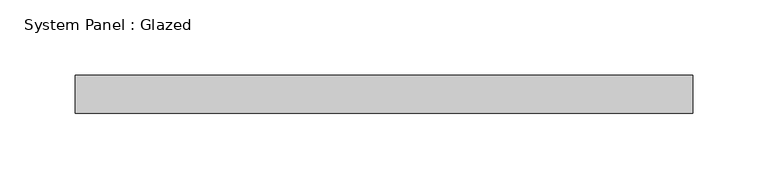
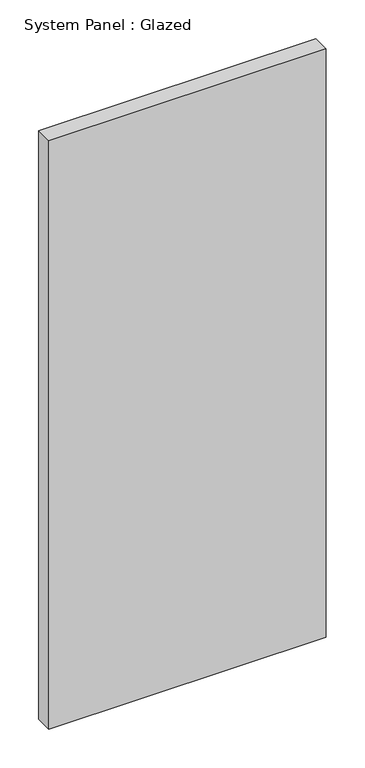
"""IFC4 building model written with IfcOpenShell, lengths in millimetres: plate geometry, System Panel : Glazed."""

from ifc_helpers import new_model, si_unit, origin, origin_with_axes, place, context, project, spatial, polyline, outline, extrude, source, transform, mapped, element, save


def system_panel_glazed_ad989134(model_context):
    return source(origin(), model_context, "Body", "SweptSolid", [
        extrude(outline(polyline([(205.3166667, 19.05), (-205.3166667, 19.05), (-205.3166667, 44.45), (205.3166667, 44.45), (205.3166667, 19.05)])), origin_with_axes(), (0.0, 0.0, 1.0), 920.75),
    ])


if __name__ == "__main__":
    model = new_model("IFC4")
    model_context = context("Model", 3, world=origin())
    ifc_project = project(units=[si_unit("LENGTHUNIT", "METRE", prefix="MILLI")], contexts=[model_context])
    site = spatial("IfcSite", under=ifc_project)
    building = spatial("IfcBuilding", under=site)
    placement = place(None, origin())
    system_panel_glazed_shape = system_panel_glazed_ad989134(model_context)
    element("IfcPlate", 1, ObjectType="System Panel : Glazed", at=placement, inside=building, context=model_context, shape_type="MappedRepresentation", body=[
        mapped(system_panel_glazed_shape, transform((0.0, 0.0, 0.0), x_axis=(1.0, 0.0, 0.0), y_axis=(0.0, 1.0, 0.0), z_axis=(0.0, 0.0, 1.0))),
    ])
    save(model, "model.ifc")

# Revit data of these elements
# Type "System Panel : Glazed"
#   Construction Type Id = "GSP4R"
#   Analytic Construction = "1/8 in Pilkington single glazing"
#   Visual Light Transmittance = 0.9
#   Solar Heat Gain Coefficient = 0.86
#   Heat Transfer Coefficient (U) = 1.18115 BTU/(h·ft²·°F)
#   Define Thermal Properties by = 1
# Element 1 (IfcPlate, "System Panel : Glazed")
#   Materials on its faces: "Glass"
# Materials
#   "Glass": class "Glass", colour RGB 0 128 192, transparency 0.75, Description = "Soda Lime Glass", Cost = 0
